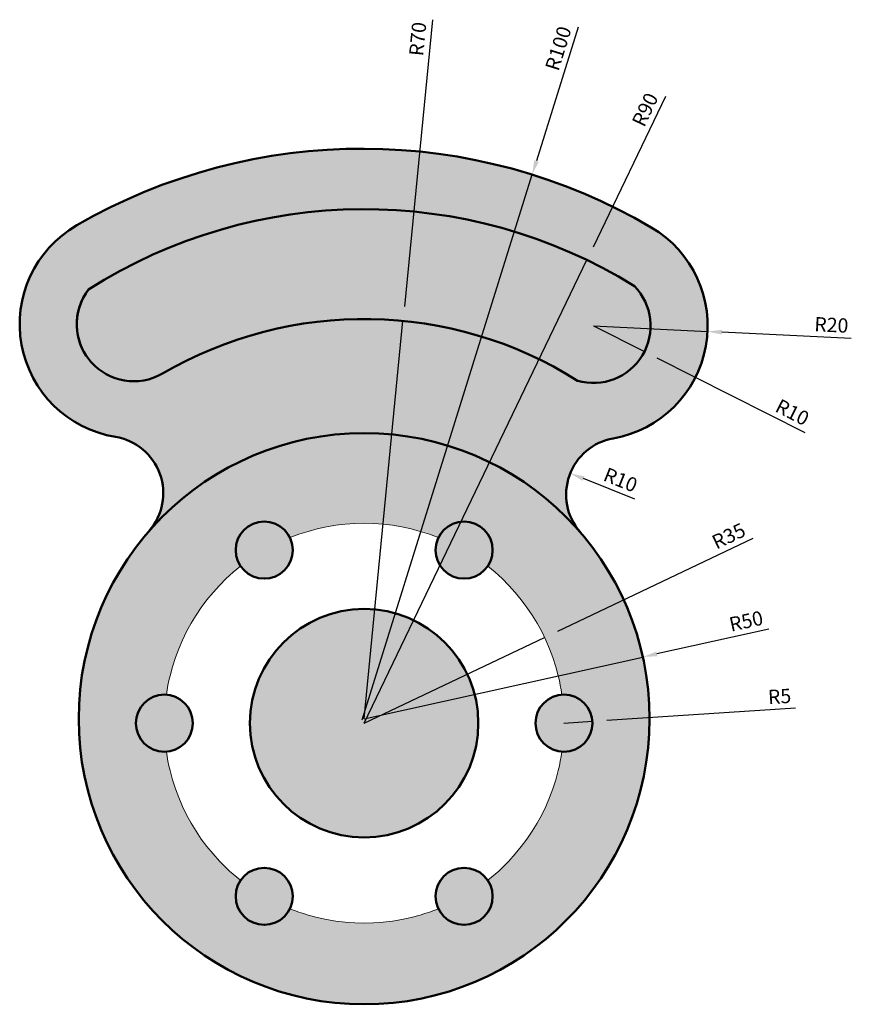
# Model space of a CAD drawing. Units: millimetres. Extents: x 2937 to 3083, y 1623 to 1796.
import ezdxf

# ---------------------------------------------------------------- set-up
doc = ezdxf.new("R2010")
doc.units = ezdxf.units.MM
doc.linetypes.add('CENTER', pattern=[50.8, 31.75, -6.35, 6.35, -6.35])
for name, color, linetype, lineweight in [('M-CNTR', 4, 'CENTER', 18), ('M-DIMS', 2, 'Continuous', 25), ('M-HATC', 8, 'Continuous', 18), ('M-OUTL', 7, 'Continuous', 50)]:
    doc.layers.add(name, color=color, linetype=linetype, lineweight=lineweight)
doc.styles.get("Standard").update_dxf_attribs({"font": 'arial.ttf'})
doc.dimstyles.new('ISO-25', dxfattribs={"dimtxt": 2.5, "dimasz": 2.5, "dimexe": 1.25, "dimexo": 0.625, "dimtad": 1, "dimtxsty": 'Standard', "dimcen": 2.5, "dimadec": 0, "dimazin": 0, "dimtfac": 1, "dimtmove": 0, "dimatfit": 3, "dimfxl": 1, "dimarcsym": 0})

# ---------------------------------------------------------------- blocks, each defined once
blk = doc.blocks.new('*D1')
at = {"layer": 'Defpoints', "color": 0, "transparency": 16777216}
for p in [(3026.77, 1768.38), (2997, 1672.92)]:
    blk.add_point(p, dxfattribs=at)
at = {"layer": 'M-DIMS', "color": 0, "lineweight": -2, "transparency": 16777216}
for p, q in [((3034.83, 1794.19), (3027.52, 1770.77)), ((2997, 1672.92), (3026.77, 1768.38))]:
    blk.add_line(p, q, dxfattribs=at)
at = {"layer": 'M-DIMS', "color": 0, "transparency": 16777216}
blk.add_solid([(3027.12, 1770.89), (3027.92, 1770.64), (3026.77, 1768.38)], dxfattribs=at)
at = {"layer": 'M-DIMS', "color": 0, "transparency": 16777216, "insert": (3031.65, 1790.39), "char_height": 2.5, "attachment_point": 5, "rotation": 72.6766}
blk.add_mtext('R100', dxfattribs=at)
blk = doc.blocks.new('*D2')
at = {"layer": 'Defpoints', "color": 0, "transparency": 16777216}
for p in [(3036.34, 1753.44), (2997.34, 1672.33)]:
    blk.add_point(p, dxfattribs=at)
at = {"layer": 'M-DIMS', "color": 0, "lineweight": -2, "transparency": 16777216}
for p, q in [((3050.1, 1782.05), (3037.43, 1755.69)), ((2997.34, 1672.33), (3036.34, 1753.44))]:
    blk.add_line(p, q, dxfattribs=at)
at = {"layer": 'M-DIMS', "color": 0, "transparency": 16777216}
blk.add_solid([(3037.05, 1755.87), (3037.8, 1755.51), (3036.34, 1753.44)], dxfattribs=at)
at = {"layer": 'M-DIMS', "color": 0, "transparency": 16777216, "insert": (3046.83, 1779.62), "char_height": 2.5, "attachment_point": 5, "rotation": 64.3152}
blk.add_mtext('R90', dxfattribs=at)
blk = doc.blocks.new('*D3')
at = {"layer": 'Defpoints', "color": 0, "transparency": 16777216}
for p in [(3037.5, 1741.9), (3057.48, 1740.91)]:
    blk.add_point(p, dxfattribs=at)
at = {"layer": 'M-DIMS', "color": 0, "lineweight": -2, "transparency": 16777216}
for p, q in [((3037.5, 1741.9), (3057.48, 1740.91)), ((3082.67, 1739.67), (3059.98, 1740.79))]:
    blk.add_line(p, q, dxfattribs=at)
at = {"layer": 'M-DIMS', "color": 0, "transparency": 16777216}
blk.add_solid([(3060, 1741.21), (3059.96, 1740.38), (3057.48, 1740.91)], dxfattribs=at)
at = {"layer": 'M-DIMS', "color": 0, "transparency": 16777216, "insert": (3079.16, 1741.75), "char_height": 2.5, "attachment_point": 5, "rotation": 357.1683}
blk.add_mtext('R20', dxfattribs=at)
blk = doc.blocks.new('*D4')
at = {"layer": 'Defpoints', "color": 0, "transparency": 16777216}
for p in [(3037.5, 1741.9), (3046.43, 1737.39)]:
    blk.add_point(p, dxfattribs=at)
at = {"layer": 'M-DIMS', "color": 0, "lineweight": -2, "transparency": 16777216}
for p, q in [((3037.5, 1741.9), (3046.43, 1737.39)), ((3074.56, 1723.15), (3048.66, 1736.26))]:
    blk.add_line(p, q, dxfattribs=at)
at = {"layer": 'M-DIMS', "color": 0, "transparency": 16777216}
blk.add_solid([(3048.85, 1736.63), (3048.47, 1735.89), (3046.43, 1737.39)], dxfattribs=at)
at = {"layer": 'M-DIMS', "color": 0, "transparency": 16777216, "insert": (3072.2, 1726.48), "char_height": 2.5, "attachment_point": 5, "rotation": 333.1617}
blk.add_mtext('R10', dxfattribs=at)
blk = doc.blocks.new('*D5')
at = {"layer": 'Defpoints', "color": 0, "transparency": 16777216}
for p in [(3028.95, 1687.34), (2997.34, 1672.33)]:
    blk.add_point(p, dxfattribs=at)
at = {"layer": 'M-DIMS', "color": 0, "lineweight": -2, "transparency": 16777216}
for p, q in [((3065.42, 1704.66), (3031.21, 1688.41)), ((2997.34, 1672.33), (3028.95, 1687.34))]:
    blk.add_line(p, q, dxfattribs=at)
at = {"layer": 'M-DIMS', "color": 0, "transparency": 16777216}
blk.add_solid([(3031.03, 1688.79), (3031.39, 1688.04), (3028.95, 1687.34)], dxfattribs=at)
at = {"layer": 'M-DIMS', "color": 0, "transparency": 16777216, "insert": (3061.33, 1704.82), "char_height": 2.5, "attachment_point": 5, "rotation": 25.3982}
blk.add_mtext('R35', dxfattribs=at)
blk = doc.blocks.new('*D6')
at = {"layer": 'Defpoints', "color": 0, "transparency": 16777216}
for p in [(3033.44, 1716.08), (3042.72, 1712.36)]:
    blk.add_point(p, dxfattribs=at)
at = {"layer": 'M-DIMS', "color": 0, "lineweight": -2, "transparency": 16777216}
blk.add_line((3044.77, 1711.53), (3035.76, 1715.15), dxfattribs=at)
at = {"layer": 'M-DIMS', "color": 0, "transparency": 16777216}
blk.add_solid([(3035.91, 1715.54), (3035.6, 1714.76), (3033.44, 1716.08)], dxfattribs=at)
at = {"layer": 'M-DIMS', "color": 0, "transparency": 16777216, "insert": (3042.13, 1714.64), "char_height": 2.5, "attachment_point": 5, "rotation": 338.1453}
blk.add_mtext('R10', dxfattribs=at)
blk = doc.blocks.new('*D7')
at = {"layer": 'Defpoints', "color": 0, "transparency": 16777216}
for p in [(3032.34, 1672.33), (3037.33, 1672.66)]:
    blk.add_point(p, dxfattribs=at)
at = {"layer": 'M-DIMS', "color": 0, "lineweight": -2, "transparency": 16777216}
for p, q in [((3072.88, 1674.98), (3039.82, 1672.82)), ((3032.34, 1672.33), (3037.33, 1672.66))]:
    blk.add_line(p, q, dxfattribs=at)
at = {"layer": 'M-DIMS', "color": 0, "transparency": 16777216}
blk.add_solid([(3039.79, 1673.23), (3039.85, 1672.4), (3037.33, 1672.66)], dxfattribs=at)
at = {"layer": 'M-DIMS', "color": 0, "transparency": 16777216, "insert": (3070.12, 1676.7), "char_height": 2.5, "attachment_point": 5, "rotation": 3.7416}
blk.add_mtext('R5', dxfattribs=at)
blk = doc.blocks.new('*D8')
at = {"layer": 'Defpoints', "color": 0, "transparency": 16777216}
for p in [(3046.15, 1683.92), (2997.34, 1673.11)]:
    blk.add_point(p, dxfattribs=at)
at = {"layer": 'M-DIMS', "color": 0, "lineweight": -2, "transparency": 16777216}
for p, q in [((3068.24, 1688.82), (3048.59, 1684.46)), ((2997.34, 1673.11), (3046.15, 1683.92))]:
    blk.add_line(p, q, dxfattribs=at)
at = {"layer": 'M-DIMS', "color": 0, "transparency": 16777216}
blk.add_solid([(3048.5, 1684.87), (3048.68, 1684.06), (3046.15, 1683.92)], dxfattribs=at)
at = {"layer": 'M-DIMS', "color": 0, "transparency": 16777216, "insert": (3064.31, 1689.89), "char_height": 2.5, "attachment_point": 5, "rotation": 12.489}
blk.add_mtext('R50', dxfattribs=at)
blk = doc.blocks.new('*D9')
at = {"layer": 'Defpoints', "color": 0, "transparency": 16777216}
for p in [(3004.14, 1742.78), (2997.34, 1673.11)]:
    blk.add_point(p, dxfattribs=at)
at = {"layer": 'M-DIMS', "color": 0, "lineweight": -2, "transparency": 16777216}
for p, q in [((3009.28, 1795.51), (3004.38, 1745.27)), ((2997.34, 1673.11), (3004.14, 1742.78))]:
    blk.add_line(p, q, dxfattribs=at)
at = {"layer": 'M-DIMS', "color": 0, "transparency": 16777216}
blk.add_solid([(3003.96, 1745.31), (3004.79, 1745.23), (3004.14, 1742.78)], dxfattribs=at)
at = {"layer": 'M-DIMS', "color": 0, "transparency": 16777216, "insert": (3007.04, 1792.1), "char_height": 2.5, "attachment_point": 5, "rotation": 84.4247}
blk.add_mtext('R70', dxfattribs=at)
blk = doc.blocks.new('HOLE-D10')
blk.add_circle((5, 5), 5)

msp = doc.modelspace()

# ---------------------------------------------------------------- hatches: boundary and pattern name
at = {"layer": 'M-HATC'}
h = msp.add_hatch(color=256, dxfattribs=at)
h.dxf.hatch_style = 1
h.set_gradient(color1=(0, 255, 0), color2=(255, 255, 0), tint=1)
h.paths.add_polyline_path([(3047.631, 1759.15, 0.2699134), (2946.998, 1759.518, 0.7048359), (2953.769, 1722.46, -0.5882124), (2959.685, 1706.011, -0.455712), (3035.154, 1705.818, -0.5822859), (3040.98, 1722.207, 0.6974288)])
h.paths.add_polyline_path([(2961.993, 1733.534), (2961.991, 1733.533, -0.8206995), (2949.07, 1748.292, -0.2875228), (3044.672, 1748.875, -0.7706997), (3034.701, 1732.304, 0.2800825)], flags=16)
h.paths.add_polyline_path([(2947.336, 1673.111, 1), (3047.336, 1673.111, 1)])
h.paths.add_polyline_path([(3010.339, 1704.825, -0.7961204), (3019.836, 1702.64, -0.1498795), (3018.977, 1699.837, -0.1926413), (3031.979, 1677.317, -0.4353108), (3037.336, 1672.329, -0.4353108), (3031.979, 1667.342, -0.1926413), (3018.977, 1644.822, -0.1498795), (3019.836, 1642.019, -0.7961204), (3010.339, 1639.834, -0.1926413), (2984.334, 1639.834, -0.7961204), (2974.836, 1642.019, -0.1498795), (2975.696, 1644.822, -0.1926413), (2962.693, 1667.342, -0.4353108), (2957.336, 1672.329, -0.4353108), (2962.693, 1677.317, -0.1926413), (2975.696, 1699.837, -0.1498795), (2974.836, 1702.64, -0.7961204), (2984.334, 1704.825, -0.1926413)], flags=16)
h.paths.add_polyline_path([(3017.336, 1672.329, -1), (2977.336, 1672.329, -1)], flags=0)
h.paths.add_polyline_path([(3009.836, 1702.64, -0.1135111), (3010.339, 1704.825, 0.1926413), (2984.334, 1704.825, -0.1135111), (2984.836, 1702.64, -0.7393127), (2975.696, 1699.837, 0.1926413), (2962.693, 1677.317, -0.3934265), (2967.336, 1672.329, -0.3934265), (2962.693, 1667.342, 0.1926413), (2975.696, 1644.822, -0.7393127), (2984.836, 1642.019, -0.1135111), (2984.334, 1639.834, 0.1926413), (3010.339, 1639.834, -0.1135111), (3009.836, 1642.019, -0.7393127), (3018.977, 1644.822, 0.1926413), (3031.979, 1667.342, -0.3934265), (3027.336, 1672.329, -0.3934265), (3031.979, 1677.317, 0.1926413), (3018.977, 1699.837, -0.7393127)], flags=0)
h = msp.add_hatch(color=256, dxfattribs=at)
h.dxf.hatch_style = 1
h.set_gradient(color1=(255, 0, 0), color2=(255, 255, 0), tint=1)
h.paths.add_polyline_path([(2977.336, 1672.329, 1), (3017.336, 1672.329, 1)])
h.paths.add_polyline_path([(2974.836, 1702.64, 1), (2984.836, 1702.64, 1)])
h.paths.add_polyline_path([(3019.836, 1702.64, 1), (3009.836, 1702.64, 1)])
h.paths.add_polyline_path([(3037.336, 1672.329, 1), (3027.336, 1672.329, 1)])
h.paths.add_polyline_path([(3009.836, 1642.019, 1), (3019.836, 1642.019, 1)])
h.paths.add_polyline_path([(2974.836, 1642.019, 1), (2984.836, 1642.019, 1)])
h.paths.add_polyline_path([(2957.336, 1672.329, 1), (2967.336, 1672.329, 1)])
h.paths.add_polyline_path([(2949.07, 1748.292, 0.82329), (2962.04, 1733.561, -0.2798721), (3034.701, 1732.304, 0.7706997), (3044.672, 1748.875, 0.2875228)])

# ---------------------------------------------------------------- linework, layer by layer
at = {"layer": 'M-CNTR'}
for start, end in [(68.19209, 111.80791), (128.19209, 171.80791), (8.19209, 51.80791), (188.19209, 231.80791), (308.19209, 351.80791), (248.19209, 291.80791)]:
    msp.add_arc((2997.336, 1672.329), 35, start, end, dxfattribs=at)
at = {"layer": 'M-OUTL'}
msp.add_line((2961.991, 1733.533), (2961.993, 1733.534), dxfattribs=at)
for centre, radius in [((2997.336, 1673.111), 50), ((2997.336, 1672.329), 20)]:
    msp.add_circle(centre, radius, dxfattribs=at)
for centre, radius, start, end in [((2996.998, 1672.916), 100, 59.5802, 120), ((2997.336, 1672.329), 90, 58.26725, 122.43185), ((2956.998, 1742.198), 20, 120, 260.71022), ((3037.504, 1741.903), 20, 280.00809, 59.5802), ((2956.998, 1742.198), 10, 142.45011, 299.95294), ((2956.998, 1742.198), 10, 142.45011, 213.58332), ((3037.504, 1741.903), 10, 253.72277, 44.20849), ((2997.336, 1673.111), 70, 57.7376, 120.32413), ((2952.155, 1712.591), 10, 318.85194, 80.71022), ((3042.718, 1712.359), 10, 100.00809, 220.85464)]:
    msp.add_arc(centre, radius, start, end, dxfattribs=at)

# ---------------------------------------------------------------- block references
for p in [(2974.836, 1697.64), (3009.836, 1697.64), (2957.336, 1667.329), (3027.336, 1667.329), (2974.836, 1637.018), (3009.836, 1637.018)]:
    msp.add_blockref('HOLE-D10', p, dxfattribs=at)

# ---------------------------------------------------------------- dimensions: what is measured, and where the dimension line sits
at = {"layer": 'M-DIMS'}
for center, mpoint, picture, middle in [((2997.336, 1673.111), (3004.136, 1742.78), '*D9', (3008.933, 1791.919)), ((2996.998, 1672.916), (3026.774, 1768.38), '*D1', (3033.462, 1789.82)), ((2997.336, 1672.329), (3036.344, 1753.437), '*D2', (3048.541, 1778.797)), ((3037.504, 1741.903), (3057.48, 1740.915), '*D3', (3079.066, 1739.847)), ((3037.504, 1741.903), (3046.427, 1737.388), '*D4', (3071.342, 1724.782)), ((3042.718, 1712.359), (3033.437, 1716.082), '*D6', (3041.426, 1712.878)), ((2997.336, 1672.329), (3028.953, 1687.341), '*D5', (3062.148, 1703.102)), ((2997.336, 1673.111), (3046.153, 1683.923), '*D8', (3064.722, 1688.036)), ((3032.336, 1672.329), (3037.326, 1672.656), '*D7', (3070.239, 1674.808))]:
    dim = msp.add_radius_dim(center=center, mpoint=mpoint, dimstyle='ISO-25', override={"dimclrd": 0, "dimclre": 0, "dimclrt": 0}, dxfattribs=at)
    dim.commit()
    dim.dimension.update_dxf_attribs({"geometry": picture, "text_midpoint": middle, "dimtype": 164})

doc.saveas('drawing.dxf')
